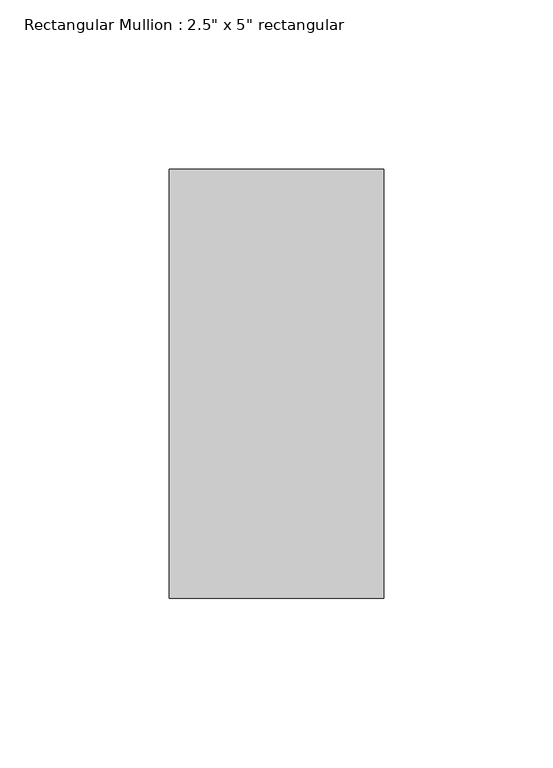
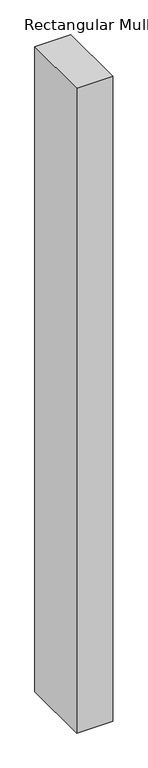
"""IFC4 building model written with IfcOpenShell, lengths in millimetres: member geometry."""

from ifc_helpers import new_model, si_unit, frame, origin, place, context, project, spatial, polyline, outline, extrude, source, transform, mapped, element, save


def member_31fee25f(model_context):
    return source(origin(), model_context, "Body", "SweptSolid", [
        extrude(outline(polyline([(31.75, 63.5), (31.75, -63.5), (-31.75, -63.5), (-31.75, 63.5), (31.75, 63.5)])), frame((0.0, 0.0, -1200.6384615), z_axis=(0.0, 0.0, 1.0), x_axis=(1.0, 0.0, 0.0)), (0.0, 0.0, 1.0), 1200.6384615),
    ])


if __name__ == "__main__":
    model = new_model("IFC4")
    model_context = context("Model", 3, world=origin())
    ifc_project = project(units=[si_unit("LENGTHUNIT", "METRE", prefix="MILLI")], contexts=[model_context])
    site = spatial("IfcSite", under=ifc_project)
    building = spatial("IfcBuilding", under=site)
    placement = place(None, origin())
    member_shape = member_31fee25f(model_context)
    element("IfcMember", 1, ObjectType="Rectangular Mullion : 2.5\" x 5\" rectangular", at=placement, inside=building, context=model_context, shape_type="MappedRepresentation", body=[
        mapped(member_shape, transform((0.0, 0.0, 0.0), x_axis=(1.0, 0.0, 0.0), y_axis=(0.0, 1.0, 0.0), z_axis=(0.0, 0.0, 1.0))),
    ])
    save(model, "model.ifc")

# Revit data of these elements
# Type "Rectangular Mullion : 2.5\" x 5\" rectangular"
#   built-in parameter 1007304 = 0.416667 (stored number, unit not read)
#   built-in parameter 1007301 = 0.104167 (stored number, unit not read)
#   built-in parameter 1007300 = 0.104167 (stored number, unit not read)
# Element 1 (IfcMember, "Rectangular Mullion : 2.5\" x 5\" rectangular")
#   Materials on its faces: "Aluminum"
# Materials
#   "Aluminum": class "Metal", colour RGB 247 247 247, transparency 0, Description = "Aluminum 6061", Cost = 0
